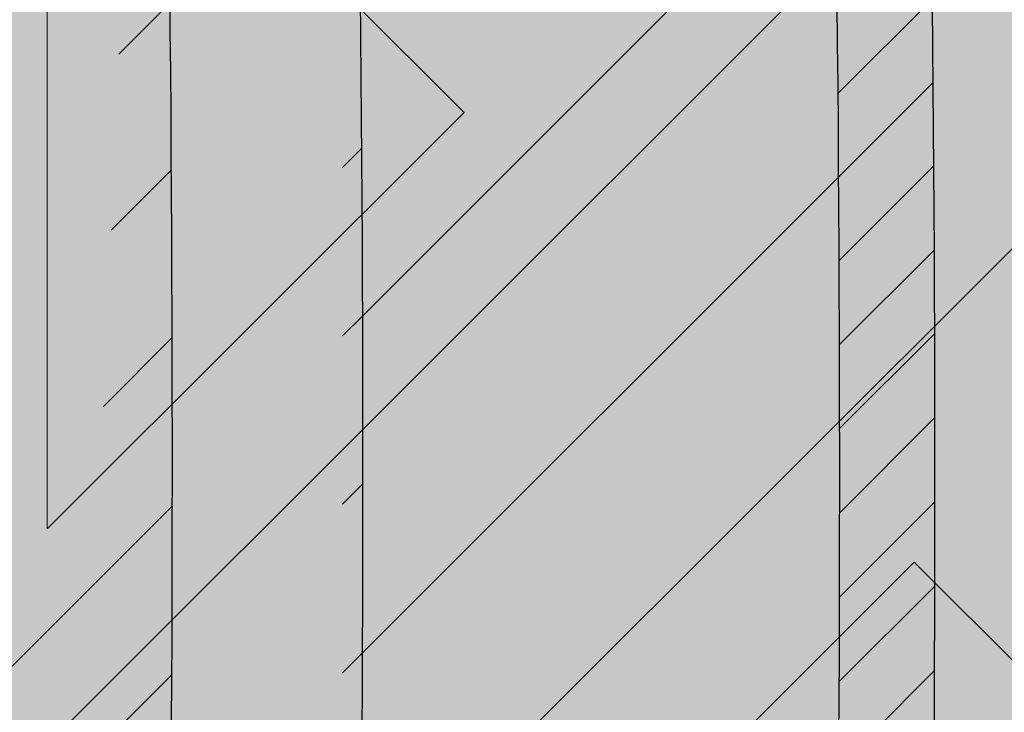
# Model space of a CAD drawing. Units: inches. Extents: x 844 to 2234, y 346 to 1084.
# Tile 11 of 93: x 1124.948 to 1126.594, y 693.702 to 694.861. Entities that reach past the tile are written whole.
import ezdxf

# ---------------------------------------------------------------- set-up
doc = ezdxf.new("R2010")
doc.units = ezdxf.units.IN
doc.header["$MEASUREMENT"] = 0
for name, color, linetype, lineweight in [('A-ANNO-DIMS', 2, 'Continuous', 18), ('furniture', 8, 'Continuous', 18), ('RA-AP-01$0$INT', 35, 'Continuous', 5)]:
    doc.layers.add(name, color=color, linetype=linetype, lineweight=lineweight)
doc.layers.add('RA-AP-01$0$FURN', color=3, linetype='Continuous')
doc.layers.add('RA-AP-01$0$WOOD', color=64, linetype='Continuous')
doc.styles.get("Standard").update_dxf_attribs({"font": 'arial.ttf'})
doc.dimstyles.get("Standard").update_dxf_attribs({"dimtxt": 6, "dimasz": 3, "dimexe": 0.18, "dimexo": 0.0625, "dimgap": 0.09, "dimtad": 0, "dimtih": 1, "dimtoh": 1, "dimdec": 1, "dimzin": 0, "dimdsep": 46, "dimlunit": 3, "dimtxsty": 'Standard', "dimblk": 'ARCHTICK', "dimcen": 0.09, "dimadec": 0, "dimazin": 0, "dimtfac": 1, "dimtdec": 1, "dimtofl": 0, "dimtmove": 0, "dimatfit": 3, "dimfxl": 1, "dimtolj": 1, "dimtzin": 0, "dimarcsym": 0})

# ---------------------------------------------------------------- blocks, each defined once
blk = doc.blocks.new('A$C18D01794')
at = {"layer": 'RA-AP-01$0$INT'}
h = blk.add_hatch(color=256, dxfattribs=at)
h.paths.add_polyline_path([(4.585917135068449, -6.356712009588271), (4.555206456959269, -6.35671200958746), (4.555206456959137, -6.387422687716308), (4.874495778835233, -6.706712009592356), (4.90520645695423, -6.676001331474049)])
h.paths.add_polyline_path([(5.255206456948813, -6.387422687716306), (5.255206456948682, -6.356712009605972), (5.224495778822613, -6.356712009605161), (4.905206456953498, -6.676001331474273), (4.935917135072151, -6.706712009592924)])
h.paths.add_polyline_path([(4.935917135072559, -6.706712009592068), (4.905206456953564, -6.737422687710376), (5.255206456951813, -7.087422687708613), (5.255206456951549, -7.026001331471008)])
h.paths.add_polyline_path([(4.555206456956399, -7.026001331471013), (4.555206456956134, -7.087422687708616), (4.905206456953821, -6.737422687710943), (4.874495778835166, -6.70671200959229)])
h = blk.add_hatch(color=256, dxfattribs=at)
h.paths.add_polyline_path([(4.585917135068448, -6.356712009588273), (4.614201406330596, -6.356712009589021), (4.668846067270487, -6.411356670531338), (4.723490728212344, -6.356712009591912), (4.771774999457151, -6.35671200959319), (4.826419660396886, -6.411356670535356), (4.862780050090322, -6.374996280843536), (4.844495778842715, -6.356712009595112), (4.862780050090411, -6.356712009595595), (4.905206456960182, -6.399138416468211), (4.947632863832445, -6.356712009597838), (4.965917135079675, -6.356712009598322), (4.947632863831759, -6.374996280845421), (4.983993253523576, -6.411356670538857), (5.038637914464627, -6.356712009600247), (5.08692218571208, -6.356712009601523), (5.141566846649976, -6.411356670541852), (5.196211507589851, -6.356712009604411), (5.224495778822615, -6.356712009605161), (4.905206456953975, -6.676001331473793)])
h.paths.add_polyline_path([(4.895206456956031, -6.637717060225675), (4.895206456958921, -6.528427738347902), (4.840561796018589, -6.583072399285802)], flags=16)
h.paths.add_polyline_path([(4.915206456955638, -6.637717060226121), (4.969851117895509, -6.583072399288678), (4.915206456957609, -6.528427738348344)], flags=16)
h.paths.add_polyline_path([(4.826419660395175, -6.568930263661755), (4.881064321335613, -6.514285602723745), (4.771774999456703, -6.514285602720857)], flags=16)
h.paths.add_polyline_path([(4.983993253519558, -6.568930263665262), (5.038637914460456, -6.514285602726792), (4.929348592581548, -6.514285602724816)], flags=16)
h.paths.add_polyline_path([(4.881064321336025, -6.494285602723742), (4.826419660397532, -6.439640941782821), (4.771774999457062, -6.494285602720859)], flags=16)
h.paths.add_polyline_path([(4.929348592582019, -6.494285602724817), (5.038637914460982, -6.494285602726792), (4.983993253522945, -6.439640941786327)], flags=16)
h.paths.add_polyline_path([(4.895206456960191, -6.480143467100443), (4.895206456962115, -6.407422687715913), (4.876922185715016, -6.389138416467584), (4.840561796021581, -6.425498806159401)], flags=16)
h.paths.add_polyline_path([(4.915206456958487, -6.480143467100889), (4.969851117899527, -6.425498806162279), (4.933490728206909, -6.389138416468043), (4.9152064569598, -6.40742268771434)], flags=16)
h.paths.add_polyline_path([(4.757632863832376, -6.480143467096812), (4.812277524772842, -6.425498806158772), (4.757632863834348, -6.370854145217844)], flags=16)
h.paths.add_polyline_path([(4.737632863832376, -6.480143467096286), (4.737632863834348, -6.370854145217375), (4.682988202893906, -6.425498806155385)], flags=16)
h.paths.add_polyline_path([(5.05278005008503, -6.480143467103376), (5.052780050087917, -6.370854145224413), (4.998135389146995, -6.425498806162908)], flags=16)
h.paths.add_polyline_path([(5.072780050085024, -6.480143467103744), (5.127424711025931, -6.42549880616527), (5.072780050087916, -6.370854145224832)], flags=16)
h.paths.add_polyline_path([(4.935917135072783, -6.706712009592292), (5.255206456948811, -6.387422687716309), (5.255206456948932, -6.415706958964177), (5.200561796010279, -6.470351619902839), (5.255206456949403, -6.524996280841948), (5.25520645694961, -6.5732805520894), (5.200561796009787, -6.627925213029239), (5.236922185702417, -6.664285602721864), (5.255206456949919, -6.646001331474357), (5.255206456949998, -6.664285602721898), (5.212780050078687, -6.706712009592262), (5.25520645695036, -6.749138416463932), (5.255206456950438, -6.767422687711313), (5.236922185702424, -6.749138416463297), (5.200561796009796, -6.785498806155928), (5.255206456950753, -6.840143467096874), (5.25520645695096, -6.888427738341682), (5.200561796010322, -6.943072399282328), (5.255206456951428, -6.997717060223427), (5.255206456951547, -7.026001331471006)])
h.paths.add_polyline_path([(5.042988202883395, -6.785498806155427), (5.097632863823085, -6.840143467095101), (5.097632863822622, -6.730854145216193)], flags=16)
h.paths.add_polyline_path([(5.028846067259663, -6.771356670531693), (5.083490728198774, -6.716712009592573), (4.974201406321001, -6.716712009593042)], flags=16)
h.paths.add_polyline_path([(5.117632863823087, -6.840143467095186), (5.172277524762331, -6.785498806155926), (5.11763286382262, -6.730854145216225)], flags=16)
h.paths.add_polyline_path([(5.08349072819877, -6.696712009593886), (5.028846067259652, -6.642067348654775), (4.974201406320998, -6.696712009593438)], flags=16)
h.paths.add_polyline_path([(5.131774999446817, -6.854285602718917), (5.186419660386065, -6.799640941779662), (5.241064321325782, -6.854285602719365)], flags=17)
h.paths.add_polyline_path([(5.131774999446228, -6.716712009592374), (5.186419660386065, -6.771356670532194), (5.222780050079488, -6.734996280838764), (5.204495778832781, -6.716712009592063)], flags=16)
h.paths.add_polyline_path([(5.097632863822613, -6.682569873970264), (5.097632863823061, -6.573280552091354), (5.042988202883383, -6.627925213031044)], flags=16)
h.paths.add_polyline_path([(5.131774999446899, -6.874285602718915), (5.241064321325809, -6.874285602719364), (5.186419660386591, -6.928930263658598)], flags=17)
h.paths.add_polyline_path([(5.131774999446226, -6.696712009594078), (5.204495778830767, -6.696712009594374), (5.22278005007868, -6.67842773834687), (5.186419660386049, -6.642067348654249)], flags=16)
h.paths.add_polyline_path([(5.11763286382262, -6.682569873970225), (5.17227752476232, -6.627925213030515), (5.117632863823064, -6.573280552091267)], flags=16)
h.paths.add_polyline_path([(5.186419660386069, -6.613783077405491), (5.241064321325754, -6.559138416465795), (5.131774999446791, -6.559138416466263)], flags=16)
h.paths.add_polyline_path([(5.131774999446872, -6.539138416466263), (5.24106432132578, -6.539138416465794), (5.186419660386554, -6.484493755526573)], flags=16)
h.paths.add_polyline_path([(5.255206456951811, -7.08742268770861), (5.255206456951895, -7.106712009588038), (4.555206456956052, -7.106712009588038), (4.555206456956136, -7.087422687708617), (4.905206456953973, -6.737422687710788)])
h.paths.add_polyline_path([(4.983993253513404, -6.8444937555241), (4.92934859257295, -6.899138416462108), (5.03863791445186, -6.899138416465014)], flags=16)
h.paths.add_polyline_path([(4.969851117889988, -6.83035161990006), (4.915206456952556, -6.775706958960171), (4.915206456949648, -6.884996280837944)], flags=16)
h.paths.add_polyline_path([(4.929348592572535, -6.919138416462105), (4.983993253511019, -6.973783077403037), (5.038637914451496, -6.919138416465012)], flags=16)
h.paths.add_polyline_path([(5.052780050074912, -6.93328055208906), (4.998135389134438, -6.987925213027088), (5.052780050072919, -7.042569873968025)], flags=16)
h.paths.add_polyline_path([(5.07278005007491, -6.933280552089588), (5.072780050072918, -7.042569873968497), (5.127424711013374, -6.987925213030498)], flags=16)
h.paths.add_polyline_path([(4.89520645695295, -6.775706958959721), (4.840561796013067, -6.830351619897157), (4.895206456950961, -6.884996280837494)], flags=16)
h.paths.add_polyline_path([(4.915206456948365, -6.933280552085403), (4.915206456946434, -7.006001331471951), (4.933490728192729, -7.024285602719066), (4.969851117886972, -6.987925213026453)], flags=16)
h.paths.add_polyline_path([(4.881064321327021, -6.899138416461022), (4.82641966038902, -6.84449375552057), (4.771774999448108, -6.899138416459029)], flags=16)
h.paths.add_polyline_path([(4.895206456950073, -6.933280552084951), (4.840561796009022, -6.987925213023558), (4.876922185700835, -7.024285602716997), (4.895206456948749, -7.006001331469487)], flags=16)
h.paths.add_polyline_path([(4.983993253510392, -7.0020673486505), (4.947632863816944, -7.038427738342319), (4.965917135064043, -7.05671200959023), (5.038637914448995, -7.056712009591555)], flags=16)
h.paths.add_polyline_path([(4.881064321326543, -6.91913841646102), (4.771774999447578, -6.919138416459031), (4.826419660385607, -6.973783077399508)], flags=16)
h.paths.add_polyline_path([(4.905206456946447, -7.014285602717636), (4.862780050074785, -7.056712009588352), (4.947632863816685, -7.056712009589775)], flags=16)
h.paths.add_polyline_path([(5.14156684663679, -7.002067348654549), (5.086922185696452, -7.056712009592438), (5.196211507574223, -7.056712009594425)], flags=16)
h.paths.add_polyline_path([(4.8264196603837, -7.002067348646972), (4.771774999442643, -7.056712009585575), (4.8444957788276, -7.056712009587508), (4.862780050075511, -7.038427738340416)], flags=16)
h.paths.add_polyline_path([(4.812277524760289, -6.98792521302292), (4.757632863822258, -6.933280552082447), (4.757632863819352, -7.042569873961408)], flags=16)
h.paths.add_polyline_path([(4.73763286382226, -6.933280552082079), (4.682988202881349, -6.987925213020536), (4.737632863819352, -7.04256987396099)], flags=16)
h.paths.add_polyline_path([(4.723490728195188, -7.056712009584289), (4.668846067257299, -7.002067348643949), (4.614201406317417, -7.056712009581383)], flags=16)
h.paths.add_polyline_path([(4.597632863829262, -6.706712009592262), (4.555206456957951, -6.664285602721896), (4.555206456958029, -6.646001331474357), (4.573490728205535, -6.664285602721864), (4.609851117898167, -6.627925213029238), (4.555206456958338, -6.573280552089402), (4.555206456958546, -6.524996280841952), (4.60985111789767, -6.470351619902839), (4.555206456959015, -6.415706958964177), (4.555206456959138, -6.387422687716309), (4.874495778835167, -6.70671200959229), (4.5552064569564, -7.026001331471015), (4.555206456956523, -6.997717060223433), (4.609851117897629, -6.94307239928233), (4.555206456956988, -6.888427738341681), (4.555206456957198, -6.840143467096881), (4.609851117898153, -6.78549880615593), (4.573490728205528, -6.749138416463297), (4.555206456957507, -6.76742268771132), (4.555206456957585, -6.749138416463933)])
h.paths.add_polyline_path([(4.712780050085332, -6.730854145216195), (4.712780050084863, -6.840143467095105), (4.767424711024555, -6.785498806155427)], flags=16)
h.paths.add_polyline_path([(4.726922185709173, -6.716712009592573), (4.781566846648288, -6.771356670531693), (4.836211507586949, -6.716712009593043)], flags=16)
h.paths.add_polyline_path([(4.692780050085327, -6.730854145216225), (4.638135389145619, -6.785498806155928), (4.692780050084865, -6.840143467095185)], flags=16)
h.paths.add_polyline_path([(4.726922185709182, -6.696712009593886), (4.836211507586949, -6.696712009593436), (4.7815668466483, -6.642067348654773)], flags=16)
h.paths.add_polyline_path([(4.678637914461726, -6.71671200959237), (4.605917135075169, -6.716712009592063), (4.587632863828464, -6.734996280838766), (4.623993253521887, -6.771356670532195)], flags=16)
h.paths.add_polyline_path([(4.712780050085336, -6.68256987397026), (4.767424711024568, -6.627925213031042), (4.71278005008489, -6.573280552091352)], flags=16)
h.paths.add_polyline_path([(4.678637914461726, -6.696712009594076), (4.623993253521899, -6.642067348654247), (4.587632863829271, -6.67842773834687), (4.605917135077185, -6.696712009594376)], flags=16)
h.paths.add_polyline_path([(4.692780050085336, -6.682569873970228), (4.692780050084889, -6.573280552091267), (4.638135389145632, -6.627925213030515)], flags=16)
h.paths.add_polyline_path([(4.623993253521885, -6.799640941779662), (4.678637914461131, -6.854285602718915), (4.56934859258217, -6.854285602719365)], flags=17)
h.paths.add_polyline_path([(4.623993253521901, -6.613783077405509), (4.678637914461158, -6.559138416466263), (4.569348592582195, -6.559138416465795)], flags=16)
h.paths.add_polyline_path([(4.678637914461051, -6.874285602718915), (4.623993253521361, -6.928930263658598), (4.569348592582143, -6.874285602719364)], flags=17)
h.paths.add_polyline_path([(4.678637914461076, -6.539138416466263), (4.623993253521399, -6.484493755526573), (4.569348592582167, -6.539138416465796)], flags=16)
h = blk.add_hatch(color=256, dxfattribs=at)
h.paths.add_polyline_path([(5.028846067259997, -6.642067348655121), (4.974201406321342, -6.696712009593783), (5.083490728199115, -6.69671200959423)])
h.paths.add_polyline_path([(4.974201406321344, -6.716712009593388), (5.028846067260004, -6.771356670532039), (5.083490728199117, -6.716712009592919)])
h.paths.add_polyline_path([(5.042988202883738, -6.785498806155768), (5.097632863823428, -6.840143467095449), (5.097632863822963, -6.73085414521654)])
h.paths.add_polyline_path([(5.117632863822961, -6.730854145216568), (5.117632863823428, -6.840143467095531), (5.172277524762674, -6.785498806156272)])
h.paths.add_polyline_path([(5.131774999446572, -6.716712009592718), (5.186419660386406, -6.77135667053254), (5.222780050079831, -6.734996280839116), (5.204495778833122, -6.716712009592409)])
h.paths.add_polyline_path([(5.236922185702764, -6.749138416463644), (5.200561796010139, -6.785498806156274), (5.255206456949971, -6.840143467096101), (5.255206456950271, -6.76742268771115)])
h.paths.add_polyline_path([(5.186419660386412, -6.799640941780006), (5.131774999447164, -6.854285602719262), (5.241064321326123, -6.854285602719711)])
h.paths.add_polyline_path([(5.131774999447238, -6.874285602719261), (5.186419660386934, -6.928930263658944), (5.241064321326153, -6.874285602719709)])
h.paths.add_polyline_path([(5.200561796010663, -6.943072399282675), (5.255206456949324, -6.997717060221329), (5.255206456949777, -6.888427738343558)])
h.paths.add_polyline_path([(5.21278005007903, -6.706712009592607), (5.255206456950223, -6.749138416463798), (5.255206456950696, -6.664285602721891)])
h.paths.add_polyline_path([(5.13177499944657, -6.696712009594424), (5.204495778831106, -6.696712009594723), (5.222780050079024, -6.678427738347219), (5.186419660386397, -6.642067348654592)])
h.paths.add_polyline_path([(5.117632863823405, -6.573280552091611), (5.117632863822955, -6.682569873970578), (5.172277524762665, -6.627925213030859)])
h.paths.add_polyline_path([(5.042988202883727, -6.627925213031387), (5.097632863822957, -6.682569873970603), (5.097632863823407, -6.573280552091697)])
h.paths.add_polyline_path([(5.131774999447135, -6.559138416466609), (5.186419660386394, -6.613783077405857), (5.241064321326097, -6.559138416466144)])
h.paths.add_polyline_path([(5.200561796010128, -6.627925213029584), (5.236922185702758, -6.664285602722211), (5.255206456950264, -6.646001331474705), (5.255206456949948, -6.573280552089752)])
h.paths.add_polyline_path([(5.186419660386895, -6.484493755526919), (5.131774999447213, -6.539138416466609), (5.241064321326127, -6.539138416466142)])
h.paths.add_polyline_path([(5.200561796010624, -6.470351619903183), (5.255206456949745, -6.524996280842298), (5.255206456949276, -6.415706958964523)])
h = blk.add_hatch(color=256, dxfattribs=at)
h.paths.add_polyline_path([(4.895206456952951, -6.77570695895972), (4.840561796013068, -6.830351619897156), (4.895206456950958, -6.884996280837495)])
h.paths.add_polyline_path([(4.915206456949649, -6.884996280837942), (4.969851117889987, -6.830351619900054), (4.915206456952556, -6.775706958960171)])
h.paths.add_polyline_path([(5.038637914451862, -6.899138416465013), (4.983993253513403, -6.8444937555241), (4.929348592572953, -6.899138416462106)])
h.paths.add_polyline_path([(4.929348592572535, -6.919138416462105), (4.983993253511018, -6.973783077403037), (5.038637914451497, -6.919138416465012)])
h.paths.add_polyline_path([(4.915206456948366, -6.933280552085397), (4.915206456946433, -7.006001331471951), (4.93349072819273, -7.024285602719068), (4.969851117886972, -6.987925213026454)])
h.paths.add_polyline_path([(5.038637914448995, -7.056712009591553), (4.983993253510389, -7.002067348650502), (4.947632863816946, -7.038427738342318), (4.965917135064043, -7.05671200959023)])
h.paths.add_polyline_path([(5.05278005007292, -7.042569873968023), (5.05278005007491, -6.933280552089059), (4.998135389134438, -6.987925213027088)])
h.paths.add_polyline_path([(5.07278005007292, -7.042569873968496), (5.127424711013374, -6.987925213030498), (5.072780050074909, -6.933280552089588)])
h.paths.add_polyline_path([(5.141566846636789, -7.002067348654547), (5.086922185696449, -7.056712009592438), (5.196211507574223, -7.056712009594425)])
h.paths.add_polyline_path([(4.947632863816688, -7.056712009589774), (4.905206456946449, -7.014285602717634), (4.862780050074784, -7.056712009588353)])
h.paths.add_polyline_path([(4.840561796009025, -6.987925213023556), (4.876922185700834, -7.024285602716997), (4.895206456948747, -7.006001331469488), (4.895206456950075, -6.933280552084953)])
h.paths.add_polyline_path([(4.88106432132654, -6.919138416461021), (4.771774999447577, -6.919138416459031), (4.826419660385606, -6.973783077399508)])
h.paths.add_polyline_path([(4.881064321327019, -6.899138416461022), (4.826419660389019, -6.844493755520571), (4.771774999448108, -6.89913841645903)])
h.paths.add_polyline_path([(4.757632863819352, -7.042569873961409), (4.812277524760284, -6.987925213022922), (4.757632863822259, -6.933280552082447)])
h.paths.add_polyline_path([(4.8264196603837, -7.002067348646974), (4.771774999442646, -7.056712009585575), (4.844495778827599, -7.05671200958751), (4.862780050075512, -7.038427738340417)])
h.paths.add_polyline_path([(4.737632863819352, -7.042569873960988), (4.737632863822258, -6.933280552082078), (4.682988202881349, -6.987925213020538)])
h.paths.add_polyline_path([(4.668846067257299, -7.002067348643952), (4.61420140631742, -7.056712009581384), (4.723490728195189, -7.056712009584292)])
for p, q in [((4.935917135072783, -6.706712009592292), (5.255206456951548, -7.026001331471007)), ((4.905206456953975, -6.737422687710788), (5.255206456951811, -7.087422687708611)), ((5.186419660386587, -6.928930263658596), (5.131774999446899, -6.874285602718915)), ((5.241064321325809, -6.874285602719364), (5.186419660386589, -6.928930263658598)), ((5.127424711013373, -6.987925213030496), (5.07278005007491, -6.933280552089588)), ((5.07278005007491, -6.933280552089588), (5.07278005007292, -7.042569873968497)), ((5.07278005007292, -7.042569873968497), (5.127424711013374, -6.987925213030498))]:
    blk.add_line(p, q, dxfattribs=at)
blk = doc.blocks.new('A$C32926AE1')
at = {"layer": 'RA-AP-01$0$FURN'}
h = blk.add_hatch(dxfattribs=at)
h.set_pattern_fill('ANSI31', color=256, scale=0.1, style=0)
h.set_pattern_definition([(45, (0, 0), (-0.0088388347648318, 0.0088388347648318), [])])
edge = h.paths.add_edge_path(flags=16)
edge.add_arc((4.904771284329206, 4.246793130718756), 0.2603971832811541, 75.22398030683196, 104.7760196931204)
edge.add_arc((4.904771284329206, 4.246793130718756), 0.2603971832811541, 75.223980306832, 104.77601969312039, ccw=False)
edge = h.paths.add_edge_path(flags=16)
edge.add_arc((4.904771284329206, 4.067062675376612), 0.2603971832811541, 255.2239803068796, 284.776019693168)
edge.add_arc((4.904771284329206, 4.067062675376612), 0.2603971832811541, 255.22398030687958, 284.77601969316805, ccw=False)
edge = h.paths.add_edge_path(flags=0)
edge.add_arc((4.904771284329206, 4.067062675376612), 0.2603971832811541, 255.2239803068796, 284.776019693168)
edge.add_arc((4.904771284329206, 4.067062675376612), 0.2603971832811541, 255.22398030687958, 284.77601969316805, ccw=False)
edge = h.paths.add_edge_path(flags=0)
edge.add_arc((4.904771284329206, 4.067062675376612), 0.2603971832811541, 255.2239803068796, 284.776019693168)
edge.add_arc((4.904771284329206, 4.067062675376612), 0.2603971832811541, 255.22398030687958, 284.77601969316805, ccw=False)
edge = h.paths.add_edge_path()
edge.add_arc((4.604388392048174, 4.588829985554312), 0.1599999999999918, 342.3781640246255, 354.4317409793762)
edge.add_arc((5.090145208887507, 4.43216705527679), 0.3503971832811637, 162.0091218307731, 180.3186872093483)
edge.add_arc((5.205154176610243, 4.588829985554953), 0.1599999999999917, 185.5682590208461, 197.6218359767349)
edge.add_arc((4.904771284329229, 4.246793130718735), 0.3503971832811761, 72.00912183053516, 107.9908781690354)
edge.add_arc((9.535952835716557, 4.28682295566602), 4.798342501046485, 178.2875002453811, 181.5576802719453)
edge.add_arc((4.719397359771122, 4.43216705527679), 0.3503971832811637, 359.6813127906516, 377.9908781692269)
edge.add_arc((9.535967292294904, 4.286822350292874), 4.778371420254705, 178.2965938931842, 181.5667745797229)
edge.add_arc((4.719397359771122, 4.43216705527679), 0.3303971832811637, 359.6813127906516, 377.9908781692269)
edge.add_arc((0.2735752763637294, 4.286822350292874), 4.7783714202547, 358.4332254202771, 361.7034061068158)
edge.add_arc((5.061434214606998, 4.732549947558029), 0.1600000000000254, 252.3781640250584, 264.4317409792362)
edge.add_arc((4.748108354051257, 4.732549947558012), 0.1600000000000541, 275.5682590208426, 287.6218359759532)
edge.add_arc((4.604388392048115, 4.588829985554317), 0.1800000000000505, 342.3567572500182, 349.3735009646207)
edge.add_arc((5.205154176610254, 4.588829985554976), 0.1800000000000069, 190.6264990356027, 197.6432427513933)
edge.add_arc((5.061434214607106, 4.732549947558013), 0.1800000000000424, 252.3567572496606, 259.3735009644582)
edge.add_arc((4.904771284329208, 4.246793130718737), 0.3303971832811676, 71.99844483668534, 108.0015551637021)
edge.add_arc((4.748108354051414, 4.732549947558045), 0.1800000000000547, 280.6264990355479, 287.6432427495938)
edge.add_arc((5.090145208887514, 4.432167055276789), 0.2803971832811691, 162.8706300666893, 180.816523289902)
edge.add_arc((4.719397359771136, 4.432167055276689), 0.2803971832811534, 359.183476710103, 377.1293699333214)
edge.add_arc((4.904771284329222, 4.246793130718737), 0.2803971832811769, 72.87063006672916, 107.1293699332334)
edge.add_arc((5.090145208887522, 4.432167055276788), 0.2603971832811776, 165.2239803068007, 180.9953123810312)
edge.add_arc((4.719397359771141, 4.432167055276699), 0.2603971832811458, 359.0046876189768, 374.7760196932087)
edge.add_arc((5.090145208887507, 4.43216705527679), 0.3303971832811637, 162.0091218307731, 180.3186872093483)
edge.add_arc((9.53595427642584, 4.285015535491528), 4.728345371032053, 178.265043920078, 181.5679956281801)
edge.add_arc((0.2735882922327999, 4.285015535491582), 4.728345371032045, 358.4320043718193, 361.7349560799204)
edge.add_arc((9.535953591267507, 4.284458026472751), 4.708343996644348, 178.2573054306777, 181.5704995759608)
edge.add_arc((0.273588977391114, 4.284458026472785), 4.708343996644358, 358.4295004240388, 361.7426945693213)
edge.add_arc((0.2735889773911131, 4.029397779622582), 4.708343996644359, 358.2573054306787, 361.5704995759613)
edge.add_arc((9.535953591267518, 4.029397779622618), 4.708343996644359, 178.4295004240391, 181.7426945693223)
edge.add_arc((0.2735882922327901, 4.028840270603786), 4.728345371032054, 358.2650439200796, 361.5679956281808)
edge.add_arc((9.53595427642584, 4.028840270603841), 4.728345371032054, 178.4320043718199, 181.7349560799219)
edge.add_arc((0.2735752763637302, 4.027033455802493), 4.778371420254699, 358.2965938931842, 361.5667745797229)
edge.add_arc((4.719397359771122, 3.881688750818578), 0.3303971832811637, 342.0091218307731, 360.3186872093484)
edge.add_arc((5.090145208887507, 3.881688750818578), 0.3303971832811637, 179.6813127906516, 197.9908781692269)
edge.add_arc((9.535967292294904, 4.027033455802493), 4.778371420254705, 178.433225420277, 181.7034061068158)
edge.add_arc((4.719397359771122, 3.881688750818578), 0.3503971832811637, 342.0091218307731, 360.3186872093484)
edge.add_arc((9.53595283571655, 4.027032850429349), 4.79834250104648, 178.4423197280546, 181.7124997546188)
edge.add_arc((4.719397359771141, 3.881688750818669), 0.2603971832811458, 345.2239803067913, 360.9953123810232)
edge.add_arc((5.090145208887522, 3.88168875081858), 0.2603971832811776, 179.0046876189687, 194.7760196931993)
edge.add_arc((4.904771284329222, 4.067062675376631), 0.2803971832811769, 252.8706300667665, 287.1293699332708)
edge.add_arc((4.719397359771136, 3.881688750818678), 0.2803971832811534, 342.8706300666787, 360.8165232898969)
edge.add_arc((5.090145208887514, 3.881688750818579), 0.2803971832811691, 179.183476710098, 197.1293699333106)
edge.add_arc((4.748108354051414, 3.581305858537323), 0.1800000000000547, 72.3567572504062, 79.37350096445199)
edge.add_arc((4.904771284329208, 4.067062675376631), 0.3303971832811676, 251.9984448362979, 288.0015551633146)
edge.add_arc((5.061434214607106, 3.581305858537355), 0.1800000000000424, 100.6264990355418, 107.6432427503394)
edge.add_arc((5.205154176610254, 3.725025820540392), 0.1800000000000069, 162.3567572486066, 169.3735009643972)
edge.add_arc((4.604388392048115, 3.725025820541051), 0.1800000000000505, 10.62649903537925, 17.64324274998182)
edge.add_arc((4.748108354051257, 3.581305858537356), 0.1600000000000541, 72.37816402404681, 84.43174097915735)
edge.add_arc((4.904771284329229, 4.067062675376632), 0.3503971832811761, 252.0091218309645, 287.9908781694648)
edge.add_arc((5.061434214606998, 3.581305858537339), 0.1600000000000254, 95.56825902076373, 107.6218359749416)
edge.add_arc((5.205154176610243, 3.725025820540414), 0.1599999999999917, 162.3781640232651, 174.4317409791539)
edge.add_arc((5.090145208887507, 3.881688750818578), 0.3503971832811637, 179.6813127906516, 197.9908781692269)
edge.add_arc((4.604388392048174, 3.725025820541056), 0.1599999999999918, 5.568259020623824, 17.62183597537444)
edge.add_arc((0.2735897329420762, 4.28682295566602), 4.798342501046482, 358.4423197280547, 361.7124997546188)
edge.add_arc((0.2735897329420691, 4.027032850429348), 4.798342501046489, 358.2875002453812, 361.5576802719453)
at = {"layer": 'RA-AP-01$0$WOOD'}
h = blk.add_hatch(color=256, dxfattribs=at)
h.dxf.hatch_style = 1
h.paths.add_polyline_path([(5.157430609644524, 4.573483066760929, -0.1009492694046607), (5.155401577623758, 4.593365984175333, -0.1842662638101597), (5.172249623284174, 4.638795604568598, 0.2056608120311276), (5.179560981299304, 4.661316324430096, 0.3614336704623542), (5.134352340494423, 4.706524965234944, 0.2056608120311297), (5.111831620632933, 4.699213607219793, -0.1842662638101113), (5.066402000239693, 4.682365561559342, -0.1055311479399994), (5.045656153913092, 4.68467289944697, 0.1567636581983829), (4.763886414745334, 4.684672899446966, -0.1055311479399895), (4.743140568418733, 4.68236556155934, -0.1842662638100833), (4.6977109480255, 4.69921360721979, 0.2056608120302612), (4.675190228164109, 4.706524965234949, 0.3614336704708441), (4.629981587358889, 4.66131632442871, 0.2056608120245944), (4.637292945374126, 4.638795604567974, -0.1842662638101024), (4.654140991034615, 4.59336598417475, -0.1009492694055169), (4.652111959013835, 4.573483066760181, 0.021410119221476), (4.629748025606143, 4.156712009541676, 0.0214101192214795), (4.652111959013809, 3.739940952323101, -0.1009492694059586), (4.654140991034615, 3.720058034908448, -0.1842662638100975), (4.637292945374126, 3.674628414515226, 0.2056608120245705), (4.629981587358889, 3.652107694654492, 0.3614336704708879), (4.675190228164113, 3.606899053848249, 0.2056608120302384), (4.697710948025501, 3.614210411863408, -0.1842662638100995), (4.743140568418738, 3.63105845752386, -0.1055311479402541), (4.763886414745388, 3.628751119636215, 0.1567636581983776), (5.045656153913137, 3.628751119636244, -0.1055311479397538), (5.066402000239692, 3.631058457523857, -0.1842662638101067), (5.111831620632931, 3.614210411863407, 0.2056608120310924), (5.134352340494417, 3.606899053848256, 0.3614336704624001), (5.179560981299307, 3.652107694653103, 0.2056608120311314), (5.172249623284175, 3.6746284145146, -0.1842662638101402), (5.155401577623758, 3.72005803490786, -0.1009492694051366), (5.15743060964455, 3.739940952322354, 0.0214101192215073), (5.179794543052287, 4.156712009541468, 0.0214101192215252)])
h.paths.add_polyline_path([(4.639748609479751, 4.156712009541513, 0.0213537860821624), (4.661970494867118, 3.741887061152232, -0.094075836301374), (4.664143710413708, 3.7196126951003, -0.1824818158568985), (4.644813765429836, 3.668037719127816, 0.2056608120245319), (4.639939526753007, 3.653023905887301, 0.3614336704710246), (4.676106439397173, 3.616856993242342, 0.2056608120302234), (4.691120252638095, 3.621731231919122, -0.1824818158602558), (4.742695228611606, 3.641061176902986, -0.1029891339458722), (4.766991894714349, 3.638256818950944, 0.156709409989566), (5.042550673941472, 3.638256818950105, -0.102989133958497), (5.066847340047078, 3.641061176902949, -0.1824818158594995), (5.118422316020358, 3.621731231919103, 0.2056608120311416), (5.133436129261316, 3.616856993242346, 0.3614336704621468), (5.169603041905217, 3.653023905886178, 0.2056608120310986), (5.164728803228477, 3.668037719127177, -0.1824818158565612), (5.145398858244737, 3.719612695099578, -0.0940758363009313), (5.147572073791232, 3.741887061151398, 0.0213537860822023), (5.169793959178681, 4.156712009541451, 0.0213537860822226), (5.147572073791203, 4.571536957931898, -0.0940758363005034), (5.145398858244737, 4.59381132398362, -0.1824818158565587), (5.164728803228476, 4.645386299956021, 0.2056608120311045), (5.169603041905216, 4.66040011319702, 0.3614336704621845), (5.133436129261313, 4.696567025840856, 0.2056608120310773), (5.118422316020359, 4.691692787164098, -0.182481815859508), (5.066847340047078, 4.67236284218025, -0.1029891339584606), (5.04255067394148, 4.675167200133092, 0.156709409989566), (4.766991894714357, 4.675167200132257, -0.1029891339458842), (4.742695228611611, 4.672362842180213, -0.1824818158602725), (4.691120252638095, 4.691692787164077, 0.2056608120302152), (4.676106439397174, 4.696567025840858, 0.3614336704710363), (4.639939526753005, 4.660400113195899, 0.2056608120245495), (4.644813765429837, 4.645386299955384, -0.1824818158568934), (4.664143710413708, 4.593811323982902, -0.0940758363009187), (4.661970494867149, 4.571536957931074, 0.021353786082177)], flags=16)
h.paths.add_polyline_path([(5.129794543052235, 4.432167055276933, -0.0141661062790638), (5.130152669293814, 4.156927903047693, -0.0141661062790647), (5.129794543052234, 3.881688750818433, -0.0785247771143638), (5.10979738006795, 3.755143611847103, 0.0945969212073497), (5.105408519571111, 3.717898134952927, 0.1043170707844957), (5.116074640131521, 3.670385395016088, 0.1043170707864965), (5.068561900193738, 3.681051515576561, 0.09459692119553), (5.031316423304057, 3.676662655080835, -0.1580239521427272), (4.778226145355827, 3.676662655080367, 0.0945969211986668), (4.740980668464973, 3.681051515576592, 0.1043170707882822), (4.693467928526415, 3.670385395015844, 0.1043170707867916), (4.704134049087309, 3.717898134953662, 0.0945969211972894), (4.69974518859162, 3.755143611844042, -0.0785247771163196), (4.679748025606343, 3.881688750818406, -0.0141661062790663), (4.679389899364763, 4.156927903047693, -0.0141661062790672), (4.679748025606343, 4.432167055276998, -0.0785247771163064), (4.699745188591625, 4.55871219425134, 0.094596921197333), (4.704134049087308, 4.595957671141738, 0.1043170707867205), (4.693467928526416, 4.643470411079523, 0.1043170707882628), (4.740980668464965, 4.632804290518776, 0.0945969211988114), (4.778226145355874, 4.637193151015016, -0.158023952142669), (5.031316423304015, 4.637193151014546, 0.0945969211956361), (5.068561900193736, 4.632804290518806, 0.1043170707864979), (5.11607464013152, 4.643470411079278, 0.1043170707844617), (5.105408519571112, 4.595957671142455, 0.0945969212074597), (5.109797380067959, 4.558712194248236, -0.0785247771143467)], flags=0)
h.paths.add_polyline_path([(5.119794532311105, 4.432259799204851, -0.0142000800617244), (5.120156169157484, 4.156927903047701, -0.0142000800617277), (5.119794532311105, 3.881596006890482, -0.0784894509520253), (5.100273383573699, 3.758192358677797, 0.0940138827242913), (5.095413455884425, 3.717477693979438, 0.0606271852308753), (5.099615656341024, 3.686844378806616, 0.0606271852322524), (5.068982341167493, 3.691046579263239, 0.0940138827010453), (5.028267676478798, 3.686186651576848, -0.1580706864508061), (4.781274892180912, 3.686186651576435, 0.0940138827026903), (4.740560227491556, 3.691046579263279, 0.0606271852339895), (4.709926912317155, 3.686844378806508, 0.0606271852329405), (4.714129112773991, 3.717477693980356, 0.094013882701304), (4.709269185087677, 3.758192358669163, -0.0784894509577193), (4.689748036347473, 3.881596006890469, -0.014200080061729), (4.689386399501094, 4.156927903047709, -0.0142000800617217), (4.689748036347473, 4.432259799204808, -0.078489450957724), (4.709269185087651, 4.555663447426125, 0.0940138827014585), (4.714129112773992, 4.596378112114996, 0.0606271852329731), (4.709926912317154, 4.62701142728886, 0.0606271852340196), (4.74056022749157, 4.622809226832087, 0.0940138827024997), (4.781274892180847, 4.627669154518912, -0.1580706864508359), (5.028267676478777, 4.627669154518526, 0.0940138827010946), (5.068982341167492, 4.622809226832129, 0.060627185232254), (5.099615656341024, 4.627011427288751, 0.0606271852308727), (5.095413455884425, 4.59637811211593, 0.0940138827241088), (5.100273383573675, 4.555663447417647, -0.0784894509520978)], flags=0)
h.paths.add_polyline_path([(5.06978912287499, 4.430218106756144, -0.014241683694547), (5.070173729147532, 4.156927903047672, -0.0142416836945458), (5.06978912287499, 3.883637699339223, -0.0800609523125196), (5.052662118612511, 3.773463122773442, 0.0526421978001116), (5.04590916754064, 3.740550867606997, 0.0526421977992423), (5.012996912374707, 3.73379791653534, -0.1583028414718258), (4.796545656286308, 3.73379791653451, 0.0526421978034211), (4.763633401117837, 3.740550867607021, 0.0526421978018622), (4.756880450045755, 3.773463122774558, -0.0800609523117106), (4.739753445783639, 3.883637699339268, -0.0142416836945435), (4.739368839511098, 4.156927903047671, -0.0142416836945477), (4.739753445783639, 4.430218106756155, -0.0800609523116345), (4.75688045004574, 4.540392683320762, 0.052642197801941), (4.763633401117837, 4.573304938488346, 0.0526421978035071), (4.796545656286361, 4.580057889560873, -0.1583028414717561), (5.012996912374669, 4.580057889560039, 0.0526421977993048), (5.04590916754064, 4.57330493848837, 0.0526421978002057), (5.052662118612529, 4.540392683321868, -0.080060952312477)], flags=0)
h.paths.add_polyline_path([(5.049789715110557, 4.43038092723357, -0.0143097550741839), (5.05018085590259, 4.156927903047715, -0.0143097550741854), (5.049789715110558, 3.883474878861827, -0.0800685599149176), (5.03362098255317, 3.779581877367999, 0.0306258898956367), (5.028241146483733, 3.758218888663947, 0.0306258898977031), (5.006878157778253, 3.75283905259408, -0.1583983521624096), (4.802664410878162, 3.752839052594731, 0.0306258898946014), (4.781301422174808, 3.758218888663924, 0.0306258898967912), (4.775921586105202, 3.779581877368794, -0.080068559914251), (4.759752853548071, 3.883474878861786, -0.0143097550741854), (4.759361712756037, 4.156927903047671, -0.0143097550741854), (4.759752853548071, 4.430380927233557, -0.0800685599142479), (4.775921586105193, 4.534273928726546, 0.0306258898968306), (4.781301422174808, 4.555636917431444, 0.0306258898945754), (4.802664410878143, 4.561016753500631, -0.1583983521624168), (5.006878157778244, 4.561016753501291, 0.0306258898977177), (5.028241146483733, 4.555636917431421, 0.0306258898958182), (5.03362098255321, 4.534273928727244, -0.080068559914796)], flags=0)
h.paths.add_polyline_path([(4.999766070382627, 4.428171244713864, -0.0143443147609634), (5.000198441819402, 4.156927903047689, -0.0143443147609612), (4.999766070382627, 3.885684561381556, -0.0784641635803329), (4.987356730658798, 3.799103304488872, -0.1506053783831347), (4.822185837999821, 3.79910330448882, -0.0784641635803318), (4.809776498276007, 3.885684561381509, -0.014344314760963), (4.809344126839227, 4.156927903047677, -0.0143443147609645), (4.809776498276007, 4.428171244713873, -0.0784641635803192), (4.822185837999822, 4.514752501606549, -0.1506053783831338), (4.987356730658798, 4.514752501606494, -0.078464163580285)], flags=0)
h.paths.add_polyline_path([(4.979755254238824, 4.42764379880488, -0.0143772539198268), (4.980205517789977, 4.156927903047693, -0.0143772539198275), (4.979755254238824, 3.886212007290489, -0.0689242507424422), (4.971183264704897, 3.815276770442801, -0.1296645318904179), (4.838359303953726, 3.815276770442746, -0.0689242507424186), (4.829787314419809, 3.886212007290419, -0.0143772539198292), (4.829337050868653, 4.156927903047653, -0.0143772539198325), (4.829787314419809, 4.427643798804946, -0.0689242507424211), (4.838359303953725, 4.498579035652621, -0.1296645318904187), (4.971183264704897, 4.498579035652565, -0.0689242507424401)], flags=0)
h = blk.add_hatch(color=256, dxfattribs=at)
h.dxf.hatch_style = 1
h.paths.add_polyline_path([(5.145398858244737, 4.59381132398362, -0.1824818158565616), (5.164728803228476, 4.645386299956021, 0.2056608120311045), (5.169603041905216, 4.66040011319702, 0.3614336704621845), (5.133436129261313, 4.696567025840856, 0.2056608120310773), (5.118422316020359, 4.691692787164098, -0.182481815859508), (5.066847340047078, 4.67236284218025, -0.1029891339584606), (5.04255067394148, 4.675167200133092, 0.156709409989566), (4.766991894714357, 4.675167200132257, -0.1029891339458842), (4.742695228611611, 4.672362842180213, -0.1824818158602725), (4.691120252638095, 4.691692787164077, 0.2056608120302152), (4.676106439397174, 4.696567025840858, 0.3614336704710363), (4.639939526753005, 4.660400113195899, 0.2056608120245495), (4.644813765429837, 4.645386299955384, -0.1824818158568934), (4.664143710413708, 4.593811323982902, -0.0940758363009187), (4.661970494867149, 4.571536957931074, 0.0213537860821772), (4.639748609479751, 4.156712009541507, 0.0213537860821625), (4.661970494867119, 3.741887061152226, -0.0940758363013071), (4.664143710413708, 3.719612695100309, -0.1824818158569294), (4.644813765429836, 3.668037719127816, 0.2056608120245319), (4.639939526753007, 3.653023905887301, 0.3614336704710246), (4.676106439397173, 3.616856993242342, 0.2056608120302234), (4.691120252638095, 3.621731231919122, -0.1824818158602558), (4.742695228611606, 3.641061176902986, -0.1029891339458722), (4.766991894714349, 3.638256818950944, 0.156709409989566), (5.042550673941472, 3.638256818950105, -0.102989133958497), (5.066847340047078, 3.641061176902949, -0.1824818158594995), (5.118422316020358, 3.621731231919103, 0.2056608120311416), (5.133436129261316, 3.616856993242346, 0.3614336704621468), (5.169603041905217, 3.653023905886178, 0.2056608120310986), (5.164728803228477, 3.668037719127177, -0.1824818158565612), (5.145398858244737, 3.719612695099578, -0.0940758363009313), (5.147572073791232, 3.741887061151398, 0.0213537860822023), (5.169793959178681, 4.156712009541451, 0.0213537860822226), (5.147572073791203, 4.571536957931898, -0.0940758363004996)])
h.paths.add_polyline_path([(5.109797380067958, 4.55871219424824, -0.0785247771143472), (5.129794543052234, 4.432167055276936, -0.0141661062790644), (5.130152669293814, 4.156927903047685, -0.014166106279066), (5.129794543052234, 3.881688750818401, -0.0785247771143517), (5.109797380067946, 3.755143611847092, 0.0945969212073132), (5.105408519571111, 3.717898134952929, 0.1043170707844995), (5.116074640131521, 3.670385395016088, 0.1043170707864965), (5.068561900193738, 3.681051515576561, 0.09459692119553), (5.031316423304057, 3.676662655080835, -0.1580239521427272), (4.778226145355827, 3.676662655080367, 0.0945969211986668), (4.740980668464973, 3.681051515576592, 0.1043170707882822), (4.693467928526415, 3.670385395015844, 0.1043170707867916), (4.704134049087309, 3.717898134953662, 0.0945969211972894), (4.69974518859162, 3.755143611844042, -0.0785247771163196), (4.679748025606343, 3.881688750818406, -0.0141661062790663), (4.679389899364763, 4.156927903047693, -0.0141661062790672), (4.679748025606343, 4.432167055276998, -0.0785247771163064), (4.699745188591625, 4.55871219425134, 0.094596921197333), (4.704134049087308, 4.595957671141738, 0.1043170707867205), (4.693467928526416, 4.643470411079523, 0.1043170707882628), (4.740980668464965, 4.632804290518776, 0.0945969211988114), (4.778226145355874, 4.637193151015016, -0.158023952142669), (5.031316423304015, 4.637193151014546, 0.0945969211956361), (5.068561900193736, 4.632804290518806, 0.1043170707864979), (5.11607464013152, 4.643470411079278, 0.1043170707844617), (5.105408519571112, 4.595957671142455, 0.0945969212074504)], flags=16)
h.paths.add_polyline_path([(5.100273383573655, 4.55566344741771, -0.0784894509521388), (5.119794532311105, 4.432259799204852, -0.0142000800617252), (5.120156169157484, 4.156927903047686, -0.014200080061726), (5.119794532311105, 3.881596006890502, -0.0784894509520446), (5.100273383573696, 3.758192358677786, 0.0940138827242721), (5.095413455884425, 3.717477693979436, 0.0606271852308692), (5.099615656341024, 3.686844378806616, 0.0606271852322522), (5.068982341167493, 3.691046579263239, 0.0940138827010453), (5.028267676478798, 3.686186651576848, -0.1580706864508061), (4.781274892180912, 3.686186651576435, 0.0940138827026903), (4.740560227491556, 3.691046579263279, 0.0606271852339895), (4.709926912317155, 3.686844378806508, 0.0606271852329405), (4.714129112773991, 3.717477693980356, 0.094013882701304), (4.709269185087677, 3.758192358669163, -0.0784894509577193), (4.689748036347473, 3.881596006890469, -0.014200080061729), (4.689386399501094, 4.156927903047709, -0.0142000800617217), (4.689748036347473, 4.432259799204808, -0.078489450957724), (4.709269185087651, 4.555663447426125, 0.0940138827014585), (4.714129112773992, 4.596378112114996, 0.0606271852329731), (4.709926912317154, 4.62701142728886, 0.0606271852340196), (4.74056022749157, 4.622809226832087, 0.0940138827024997), (4.781274892180847, 4.627669154518912, -0.1580706864508359), (5.028267676478777, 4.627669154518526, 0.0940138827010946), (5.068982341167492, 4.622809226832129, 0.060627185232254), (5.099615656341024, 4.627011427288751, 0.0606271852308727), (5.095413455884425, 4.59637811211593, 0.094013882723957)], flags=0)
h.paths.add_polyline_path([(5.04590916754064, 4.57330493848837, 0.0526421978002057), (5.052662118612529, 4.540392683321868, -0.0800609523124783), (5.06978912287499, 4.430218106756142, -0.0142416836945469), (5.070173729147532, 4.156927903047672, -0.0142416836945458), (5.06978912287499, 3.883637699339223, -0.0800609523125196), (5.052662118612511, 3.773463122773442, 0.0526421978001116), (5.04590916754064, 3.740550867606997, 0.0526421977992423), (5.012996912374707, 3.73379791653534, -0.1583028414718258), (4.796545656286308, 3.73379791653451, 0.0526421978034211), (4.763633401117837, 3.740550867607021, 0.0526421978018622), (4.756880450045755, 3.773463122774558, -0.0800609523117106), (4.739753445783639, 3.883637699339268, -0.0142416836945435), (4.739368839511098, 4.156927903047671, -0.0142416836945477), (4.739753445783639, 4.430218106756155, -0.0800609523116345), (4.75688045004574, 4.540392683320762, 0.052642197801941), (4.763633401117837, 4.573304938488346, 0.0526421978035071), (4.796545656286361, 4.580057889560873, -0.1583028414717561), (5.012996912374669, 4.580057889560039, 0.0526421977993048)], flags=0)
h.paths.add_polyline_path([(5.028241146483733, 4.555636917431422, 0.0306258898956949), (5.033620982553182, 4.534273928727329, -0.0800685599148649), (5.049789715110557, 4.430380927233569, -0.0143097550741839), (5.05018085590259, 4.156927903047715, -0.0143097550741854), (5.049789715110558, 3.883474878861827, -0.0800685599149176), (5.03362098255317, 3.779581877367999, 0.0306258898956367), (5.028241146483733, 3.758218888663947, 0.0306258898977031), (5.006878157778253, 3.75283905259408, -0.1583983521624096), (4.802664410878162, 3.752839052594731, 0.0306258898946014), (4.781301422174808, 3.758218888663924, 0.0306258898967912), (4.775921586105202, 3.779581877368794, -0.080068559914251), (4.759752853548071, 3.883474878861786, -0.0143097550741854), (4.759361712756037, 4.156927903047671, -0.0143097550741854), (4.759752853548071, 4.430380927233557, -0.0800685599142479), (4.775921586105193, 4.534273928726546, 0.0306258898968306), (4.781301422174808, 4.555636917431444, 0.0306258898945754), (4.802664410878143, 4.561016753500631, -0.1583983521624168), (5.006878157778244, 4.561016753501291, 0.0306258898977174)], flags=0)
h.paths.add_polyline_path([(4.987356730658798, 4.514752501606494, -0.0784641635803018), (4.999766070382627, 4.428171244713845, -0.0143443147609637), (5.000198441819402, 4.156927903047665, -0.0143443147609622), (4.999766070382628, 3.885684561381514, -0.0784641635802952), (4.987356730658797, 3.799103304488872, -0.1506053783831338), (4.822185837999821, 3.799103304488819, -0.0784641635803342), (4.809776498276007, 3.885684561381512, -0.0143443147609628), (4.809344126839227, 4.156927903047676, -0.0143443147609646), (4.809776498276007, 4.428171244713873, -0.0784641635803192), (4.822185837999822, 4.514752501606549, -0.1506053783831338)], flags=0)
h.paths.add_polyline_path([(4.971183264704897, 4.498579035652566, -0.0689242507424384), (4.979755254238824, 4.427643798804883, -0.0143772539198276), (4.980205517789977, 4.15692790304768, -0.0143772539198258), (4.979755254238823, 3.88621200729051, -0.0689242507424628), (4.971183264704897, 3.815276770442801, -0.129664531890417), (4.838359303953726, 3.815276770442746, -0.0689242507424186), (4.829787314419809, 3.886212007290419, -0.0143772539198292), (4.829337050868653, 4.156927903047653, -0.0143772539198325), (4.829787314419809, 4.427643798804946, -0.0689242507424211), (4.838359303953725, 4.498579035652621, -0.1296645318904187)], flags=0)
h = blk.add_hatch(dxfattribs=at)
h.set_pattern_fill('ANSI31', color=256, scale=0.05, style=0)
h.set_pattern_definition([(45, (0, 0), (-0.0044194173824159, 0.0044194173824159), [])])
h.paths.add_polyline_path([(5.130152669293814, 4.156927903047704, 0.0141661062790657), (5.129794543052234, 4.432167055276982, 0.0777827904001433), (5.110168979996553, 4.557559993161921, -0.0976515123401879), (5.105408519571111, 4.595957671142454, -0.1043170707844687), (5.116074640131522, 4.64347041107928), (5.099615656341024, 4.627011427288751, 0.0606271852308727), (5.095413455884425, 4.59637811211593, 0.0940138827241088), (5.100273383573675, 4.555663447417647, -0.0784894509520972), (5.119794532311105, 4.432259799204852, -0.0142000800617252), (5.120156169157484, 4.156927903047686, -0.014200080061726), (5.119794532311105, 3.881596006890502, -0.0784894509520446), (5.100273383573696, 3.758192358677786, 0.0940138827242721), (5.095413455884425, 3.717477693979436, 0.0606271852308692), (5.099615656341024, 3.686844378806616), (5.116074640131519, 3.67038539501609, -0.1043170707844594), (5.105408519571112, 3.717898134952912, -0.0976515123401594), (5.11016897999655, 3.756295812933435, 0.0777827904001654), (5.129794543052234, 3.881688750818409, 0.0141661062790665)])
h.paths.add_polyline_path([(5.030164222210597, 3.676291055149937, -0.0976515123472002), (5.068561900193739, 3.681051515576561, -0.1043170707864927), (5.116074640131521, 3.670385395016088), (5.099615656341024, 3.686844378806616, 0.0606271852322522), (5.068982341167493, 3.691046579263239, 0.0940138827010453), (5.028267676478798, 3.686186651576848, -0.1580706864508061), (4.781274892180912, 3.686186651576435, 0.0940138827026903), (4.740560227491556, 3.691046579263279, 0.0606271852339913), (4.709926912317154, 3.686844378806508), (4.693467928526416, 3.670385395015845, -0.1043170707882796), (4.740980668464973, 3.681051515576592, -0.0976515123427246), (4.779378346446416, 3.676291055150394, 0.156512506893803)])
h.paths.add_polyline_path([(4.689748036347473, 3.881596006890472, -0.014200080061729), (4.689386399501094, 4.156927903047712, -0.0142000800617195), (4.689748036347473, 4.432259799204768, -0.078489450957742), (4.709269185087648, 4.555663447426114, 0.0940138827014821), (4.714129112773992, 4.596378112114995, 0.0606271852329748), (4.709926912317154, 4.62701142728886), (4.693467928526414, 4.643470411079524, -0.1043170707867939), (4.704134049087309, 4.595957671141706, -0.09765151234893), (4.699373588660725, 4.557559993157876, 0.0777827903975372), (4.679748025606343, 4.432167055276987, 0.0141661062790675), (4.679389899364763, 4.156927903047675, 0.0141661062790641), (4.679748025606343, 3.88168875081843, 0.0777827903975637), (4.699373588660724, 3.756295812937497, -0.0976515123490278), (4.704134049087308, 3.717898134953629, -0.1043170707867196), (4.693467928526416, 3.670385395015845), (4.709926912317155, 3.686844378806508, 0.0606271852329413), (4.714129112773991, 3.717477693980357, 0.0940138827013084), (4.709269185087676, 3.758192358669166, -0.0784894509577192)])
h.paths.add_polyline_path([(4.779378346446434, 4.63756475094498, -0.0976515123427943), (4.740980668464964, 4.632804290518776, -0.1043170707882609), (4.693467928526416, 4.643470411079523), (4.709926912317154, 4.62701142728886, 0.0606271852340196), (4.74056022749157, 4.622809226832087, 0.0940138827024997), (4.781274892180847, 4.627669154518912, -0.1580706864508359), (5.028267676478777, 4.627669154518526, 0.0940138827010946), (5.068982341167492, 4.622809226832129, 0.060627185232254), (5.099615656341024, 4.627011427288751), (5.116074640131521, 4.643470411079279, -0.1043170707865022), (5.068561900193735, 4.632804290518806, -0.0976515123475899), (5.030164222210446, 4.637564750945479, 0.1565125068936924)])
h = blk.add_hatch(dxfattribs=at)
h.set_pattern_fill('ANSI32', color=256, scale=0.2, style=0)
h.set_pattern_definition([(45, (0, 0), (-0.0530330085889911, 0.0530330085889911), []), (45, (0.035355339, 0), (-0.0530330085889911, 0.0530330085889911), [])])
h.paths.add_polyline_path([(5.119794532311105, 4.432259799204823, 0.0777015974868765), (5.10065834347252, 4.554469821747928, -0.0968902511992216), (5.095413455884425, 4.596378112115931, -0.060627185230871), (5.099615656341024, 4.627011427288751, -0.060627185232254), (5.068982341167492, 4.622809226832129, -0.0968902512198245), (5.027074050790956, 4.628054114423209, 0.1564657949319105), (4.782468517866163, 4.628054114422785, -0.0968902512152247), (4.740560227491555, 4.622809226832088, -0.0606271852339878), (4.709926912317155, 4.627011427288859, -0.0606271852329413), (4.714129112773991, 4.596378112115011, -0.0968902512205338), (4.708884225182929, 4.554469821738175, 0.0777015974804443), (4.689748036347473, 4.43225979920482, 0.0142000800617215), (4.689386399501094, 4.156927903047726, 0.0142000800617273), (4.689748036347473, 3.88159600689052, 0.077701597480541), (4.708884225182985, 3.759385984357019, -0.096890251220082), (4.714129112773992, 3.717477693980371, -0.0606271852329731), (4.709926912317154, 3.686844378806507, -0.060627185233988), (4.740560227491554, 3.691046579263279, -0.0968902512152569), (4.782468517866175, 3.685801691672578, 0.1564657949319236), (5.027074050790988, 3.685801691672169, -0.0968902512197451), (5.068982341167491, 3.691046579263239, -0.0606271852322557), (5.099615656341024, 3.686844378806616, -0.0606271852308727), (5.095413455884425, 3.717477693979438, -0.0968902511991229), (5.100658343472507, 3.7593859843474, 0.0777015974868745), (5.119794532311105, 3.8815960068905, 0.014200080061726), (5.120156169157484, 4.156927903047685, 0.0142000800617238)])
h.paths.add_polyline_path([(5.070173729147531, 4.156927903047684, -0.0142416836945481), (5.06978912287499, 3.883637699339191, -0.0800609523125107), (5.052662118612505, 3.773463122773424, 0.0526421978000811), (5.04590916754064, 3.740550867606997, 0.0526421977993214), (5.012996912374658, 3.733797916535325, -0.1583028414717916), (4.796545656286304, 3.733797916534512, 0.0526421978034138), (4.763633401117837, 3.740550867607021, 0.0526421978018622), (4.756880450045755, 3.773463122774558, -0.0800609523117106), (4.739753445783639, 3.883637699339268, -0.0142416836945435), (4.739368839511098, 4.156927903047671, -0.0142416836945477), (4.739753445783639, 4.430218106756155, -0.0800609523116345), (4.75688045004574, 4.540392683320762, 0.052642197801941), (4.763633401117837, 4.573304938488346, 0.0526421978035071), (4.796545656286361, 4.580057889560873, -0.1583028414717561), (5.012996912374669, 4.580057889560039, 0.0526421977993048), (5.04590916754064, 4.57330493848837, 0.0526421978002057), (5.052662118612529, 4.540392683321868, -0.0800609523124783), (5.06978912287499, 4.430218106756142, -0.0142416836945463)], flags=16)
h.paths.add_polyline_path([(5.050180855902591, 4.156927903047686, -0.0143097550741856), (5.049789715110558, 3.883474878861795, -0.0800685599148126), (5.033620982553202, 3.7795818773681, 0.0306258898957837), (5.028241146483733, 3.758218888663947, 0.0306258898977031), (5.006878157778253, 3.75283905259408, -0.1583983521624096), (4.802664410878162, 3.752839052594731, 0.0306258898946014), (4.781301422174808, 3.758218888663924, 0.0306258898967912), (4.775921586105202, 3.779581877368794, -0.080068559914251), (4.759752853548071, 3.883474878861786, -0.0143097550741854), (4.759361712756037, 4.156927903047671, -0.0143097550741854), (4.759752853548071, 4.430380927233557, -0.0800685599142479), (4.775921586105193, 4.534273928726546, 0.0306258898968306), (4.781301422174808, 4.555636917431444, 0.0306258898945754), (4.802664410878143, 4.561016753500631, -0.1583983521624168), (5.006878157778244, 4.561016753501291, 0.0306258898977177), (5.028241146483733, 4.555636917431421, 0.0306258898958182), (5.03362098255321, 4.534273928727244, -0.0800685599147973), (5.049789715110557, 4.430380927233568, -0.0143097550741854)], flags=0)
h.paths.add_polyline_path([(5.000198441819402, 4.15692790304769, -0.0143443147609622), (4.999766070382627, 3.885684561381539, -0.0784641635803169), (4.987356730658798, 3.799103304488873, -0.1506053783831347), (4.822185837999821, 3.79910330448882, -0.0784641635803318), (4.809776498276007, 3.885684561381509, -0.014344314760963), (4.809344126839227, 4.156927903047677, -0.0143443147609645), (4.809776498276007, 4.428171244713873, -0.0784641635803192), (4.822185837999822, 4.514752501606549, -0.1506053783831338), (4.987356730658798, 4.514752501606494, -0.0784641635803018), (4.999766070382627, 4.428171244713845, -0.0143443147609624)], flags=0)
h.paths.add_polyline_path([(4.980205517789976, 4.156927903047707, -0.0143772539198295), (4.979755254238824, 3.886212007290466, -0.06892425074242), (4.971183264704897, 3.815276770442801, -0.129664531890417), (4.838359303953726, 3.815276770442746, -0.0689242507424186), (4.829787314419809, 3.886212007290419, -0.0143772539198292), (4.829337050868653, 4.156927903047653, -0.0143772539198325), (4.829787314419809, 4.427643798804946, -0.0689242507424211), (4.838359303953725, 4.498579035652621, -0.1296645318904187), (4.971183264704897, 4.498579035652565, -0.0689242507424418), (4.979755254238824, 4.427643798804878, -0.0143772539198259)], flags=0)
for centre, radius, start, end in [((0.2735752763637302, 4.027033455802493), 4.778371420254699, 358.2965938931842, 1.56677457972295), ((0.2735897329420691, 4.027032850429348), 4.798342501046489, 358.2875002453812, 1.557680271945363), ((0.2735875766687554, 4.025627481140981), 4.848346823659695, 358.3067023394723, 1.551844405055681), ((0.2735947217851784, 4.025627183474594), 4.85833253045422, 358.302242255809, 1.547383999763723)]:
    blk.add_arc(centre, radius, start, end, dxfattribs=at)
blk = doc.blocks.new('A$C5D2F253E')
at = {"layer": 'RA-AP-01$0$FURN', "xscale": -0.7999999999883585, "yscale": 0.7999999999883585, "zscale": 0.8, "rotation": 90}
blk.add_blockref('A$C18D01794', (-5.687757199772477, 4.75791982714071), dxfattribs=at)
at = {"layer": 'RA-AP-01$0$WOOD', "rotation": 270}
blk.add_blockref('A$C32926AE1', (-4.161339601644158, 5.73852594588169), dxfattribs=at)
blk = doc.blocks.new('_ArchTick')
at = {"color": 0, "linetype": 'ByBlock', "const_width": 0.15}
blk.add_lwpolyline([(-0.5, -0.5), (0.5, 0.5)], dxfattribs=at)
blk = doc.blocks.new('*D144')
at = {"layer": 'A-ANNO-DIMS', "color": 0, "lineweight": -2, "transparency": 16777216}
for p, q in [((1096.615948, 439.3732739999999), (1096.615948, 1074.743301)), ((1143.115948, 492.373274), (1143.115948, 1074.743301)), ((1096.615948, 1074.563301), (1102.481950728513, 1074.563301)), ((1143.115948, 1074.563301), (1137.249945271487, 1074.563301))]:
    blk.add_line(p, q, dxfattribs=at)
at = {"layer": 'Defpoints', "color": 0, "transparency": 16777216}
for p in [(1143.115948, 1074.563301), (1143.115948, 492.3107739999999), (1096.615948, 439.3107739999999)]:
    blk.add_point(p, dxfattribs=at)
at = {"layer": 'A-ANNO-DIMS', "color": 0, "lineweight": -2, "transparency": 16777216, "xscale": 3, "yscale": 3, "zscale": 3, "rotation": 180}
blk.add_blockref('_ArchTick', (1096.615948, 1074.563301), dxfattribs=at)
at = {"layer": 'A-ANNO-DIMS', "color": 0, "lineweight": -2, "transparency": 16777216, "xscale": 3, "yscale": 3, "zscale": 3}
blk.add_blockref('_ArchTick', (1143.115948, 1074.563301), dxfattribs=at)
at = {"layer": 'A-ANNO-DIMS', "color": 0, "transparency": 16777216, "insert": (1119.865948, 1074.563301), "char_height": 6, "attachment_point": 5}
blk.add_mtext('\\A1;3\'-10 1/2"', dxfattribs=at)

msp = doc.modelspace()

# ---------------------------------------------------------------- block references
at = {"layer": 'furniture', "xscale": 15.94108302203742, "yscale": 15.94108302203742, "zscale": 15.94108302203742, "rotation": 90}
msp.add_blockref('A$C5D2F253E', (1136.147844094663, 696.2584716700112), dxfattribs=at)

# ---------------------------------------------------------------- dimensions: what is measured, and where the dimension line sits
at = {"layer": 'A-ANNO-DIMS'}
dim = msp.add_linear_dim(base=(1143.115948, 1074.563301), p1=(1096.615948, 439.3107739999999), p2=(1143.115948, 492.3107739999999), dimstyle='Standard', override={"dimdec": 1, "dimlfac": 1, "dimrnd": 0, "dimzin": 1, "dimdsep": 46, "dimlunit": 4, "dimfrac": 2}, dxfattribs=at)
dim.commit()
dim.dimension.update_dxf_attribs({"geometry": '*D144', "text_midpoint": (1119.865948, 1074.563301)})

doc.saveas('drawing.dxf')
